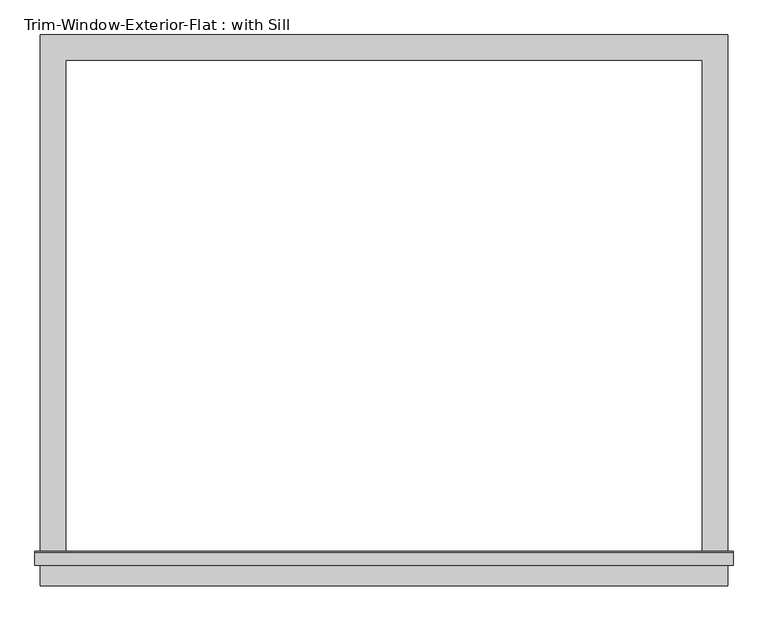
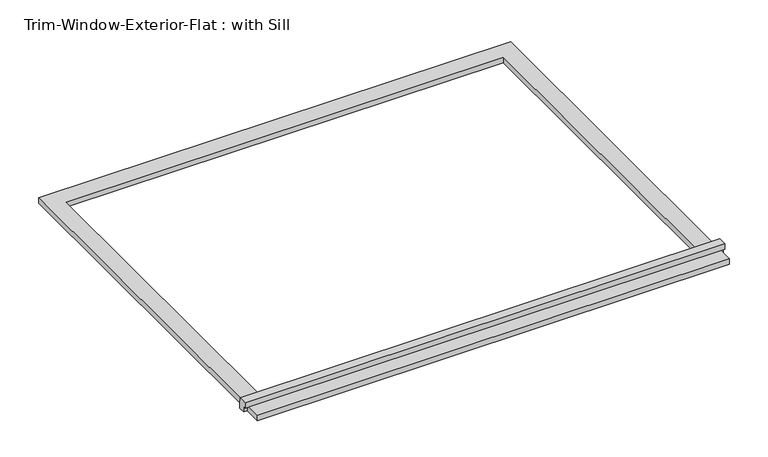
"""IFC4 building model written with IfcOpenShell, lengths in millimetres: proxy geometry, Trim-Window-Exterior-Flat : with Sill."""

from ifc_helpers import new_model, si_unit, frame, origin, origin_with_axes, place, context, project, spatial, polyline, outline, extrude, source, transform, mapped, element, save


def trim_window_exterior_flat_with_sill_f4abd27b(model_context):
    return source(origin(), model_context, "Body", "SweptSolid", [
        extrude(outline(polyline([(781.05, -1139.7823709), (781.05, -1196.9323709), (-781.05, -1196.9323709), (-781.05, -1139.7823709), (781.05, -1139.7823709)])), origin_with_axes(), (0.0, 0.0, 1.0), 19.05),
        extrude(outline(polyline([(-1149.35, 38.1), (-1120.0580645, 38.1), (-1117.6, 19.05), (-1117.6, 0.0), (-1139.7823709, 0.0), (-1139.7823709, 19.05), (-1149.35, 19.05), (-1149.35, 38.1)])), frame((-793.75, 0.0, 0.0), z_axis=(1.0, 0.0, 0.0), x_axis=(0.0, 1.0, 0.0)), (0.0, 0.0, 1.0), 1587.5),
        extrude(outline(polyline([(-781.05, 57.15), (781.05, 57.15), (781.05, -1117.6), (723.9, -1117.6), (723.9, 0.0), (-723.9, 0.0), (-723.9, -1117.6), (-781.05, -1117.6), (-781.05, 57.15)])), origin_with_axes(), (0.0, 0.0, 1.0), 19.05),
    ])


if __name__ == "__main__":
    model = new_model("IFC4")
    model_context = context("Model", 3, world=origin())
    ifc_project = project(units=[si_unit("LENGTHUNIT", "METRE", prefix="MILLI")], contexts=[model_context])
    site = spatial("IfcSite", under=ifc_project)
    building = spatial("IfcBuilding", under=site)
    placement = place(None, origin())
    trim_window_exterior_flat_with_sill_shape = trim_window_exterior_flat_with_sill_f4abd27b(model_context)
    element("IfcBuildingElementProxy", 1, Name="Trim-Window-Exterior-Flat : with Sill", ObjectType="Trim-Window-Exterior-Flat : with Sill", at=placement, inside=building, context=model_context, shape_type="MappedRepresentation", body=[
        mapped(trim_window_exterior_flat_with_sill_shape, transform((0.0, 0.0, 0.0), x_axis=(1.0, 0.0, 0.0), y_axis=(0.0, 1.0, 0.0), z_axis=(0.0, 0.0, 1.0))),
    ])
    save(model, "model.ifc")

# Revit data of these elements
# Type "Trim-Window-Exterior-Flat : with Sill"
#   Trim Width = 2.25"
#   Trim Thickness_Picture Frame = 1.25"
#   Trim Thickness_with Sill = 0.75"
#   Sill Thickness = 1.25"
#   Opening Width [instance default] = 24"
#   Opening Height [instance default] = 36"
#   Default Elevation = 48"
#   Sill = yes
#   Picture Frame = no
#   Trim Material [instance default] = none
# Element 1 (IfcBuildingElementProxy, "Trim-Window-Exterior-Flat : with Sill")
#   Opening Width = 57"
#   Opening Height = 44"
#   Trim Material = Clad - White
#   Materials on its faces: "Clad - White"
# Materials
#   "Clad - White": class "Wood", colour RGB 242 242 238, transparency 0, Cost = 0
